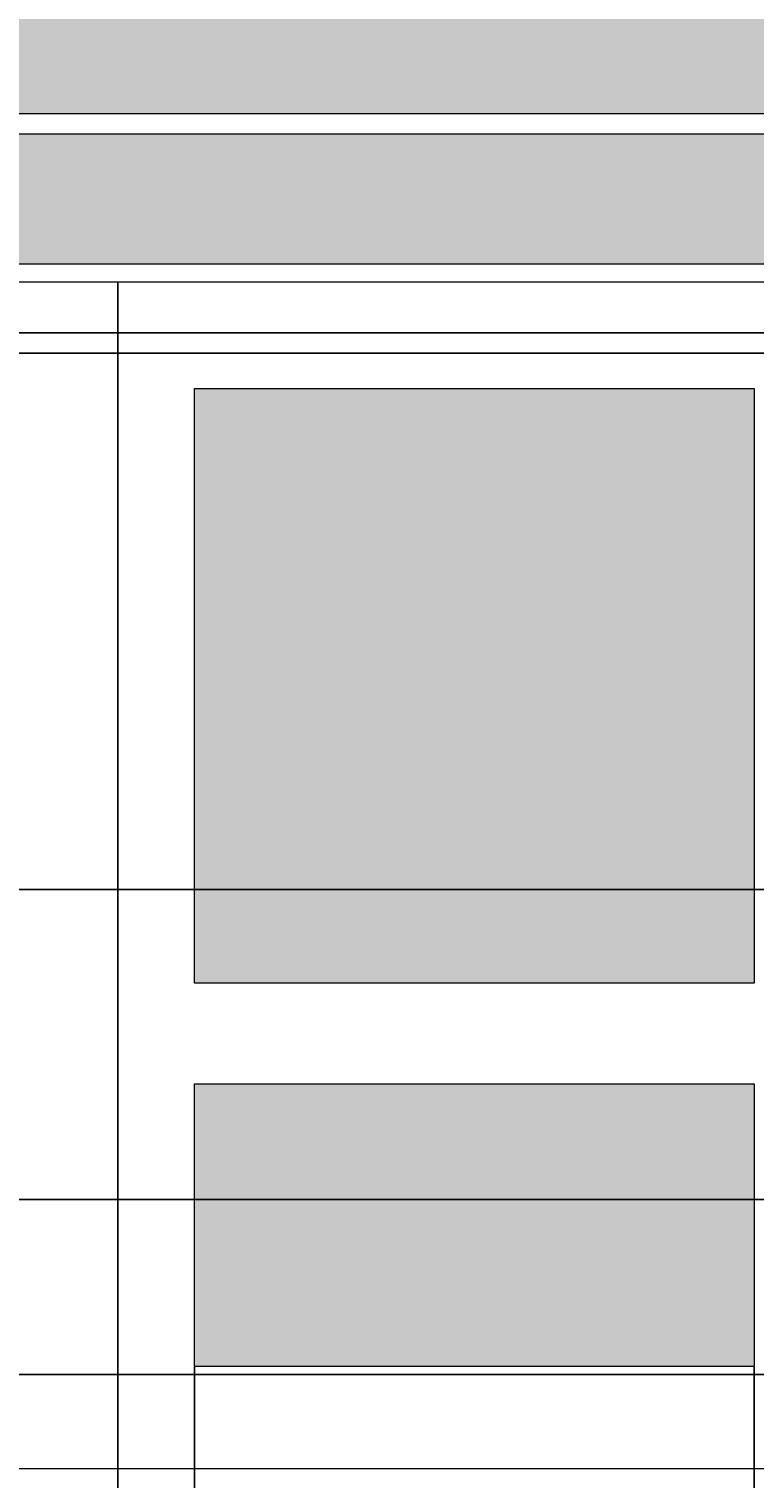
# Model space of a CAD drawing. Units: inches. Extents: x 36 to 594, y 79 to 831.
# Tile 6 of 30: x 319 to 390, y 152 to 294. Entities that reach past the tile are written whole.
import ezdxf

# ---------------------------------------------------------------- set-up
doc = ezdxf.new("R2010")
doc.units = ezdxf.units.IN
doc.header["$MEASUREMENT"] = 0
for name, color, linetype, lineweight in [('A-ANNO-DIMS', 2, 'Continuous', 18), ('A-DOOR', 3, 'Continuous', 18), ('A-ELEV-PATT', 8, 'Continuous', 13)]:
    doc.layers.add(name, color=color, linetype=linetype, lineweight=lineweight)
doc.styles.get("Standard").update_dxf_attribs({"font": 'arial.ttf'})
doc.dimstyles.get("Standard").update_dxf_attribs({"dimtxt": 0.8125, "dimasz": 0.18, "dimexe": 0.18, "dimexo": 0.0625, "dimgap": 0.09, "dimtad": 0, "dimtih": 1, "dimtoh": 1, "dimdec": 4, "dimzin": 0, "dimdsep": 46, "dimlunit": 4, "dimtxsty": 'Standard', "dimcen": 0.09, "dimadec": 0, "dimazin": 0, "dimtfac": 1, "dimtdec": 4, "dimtofl": 0, "dimtmove": 0, "dimatfit": 3, "dimfxl": 1, "dimtolj": 1, "dimtzin": 0, "dimarcsym": 0})

# ---------------------------------------------------------------- blocks, each defined once
blk = doc.blocks.new('*D74')
at = {"layer": 'A-ANNO-DIMS', "color": 0, "lineweight": -2, "transparency": 16777216}
for p, q in [((217.09, 179.42), (592.85, 179.42)), ((592.67, 179.24), (592.67, 171.32)), ((592.67, 162.39), (592.67, 170.31)), ((217.09, 162.21), (592.85, 162.21))]:
    blk.add_line(p, q, dxfattribs=at)
at = {"layer": 'A-ANNO-DIMS', "color": 0, "transparency": 16777216}
for points in [[(592.64, 179.24), (592.7, 179.24), (592.67, 179.42)], [(592.64, 162.39), (592.7, 162.39), (592.67, 162.21)]]:
    blk.add_solid(points, dxfattribs=at)
at = {"layer": 'Defpoints', "color": 0, "transparency": 16777216}
for p in [(217.03, 179.42), (592.67, 179.42), (217.03, 162.21)]:
    blk.add_point(p, dxfattribs=at)
at = {"layer": 'A-ANNO-DIMS', "color": 0, "transparency": 16777216, "insert": (592.67, 170.82), "char_height": 0.812, "attachment_point": 5}
blk.add_mtext('\\A1;17.207', dxfattribs=at)
blk = doc.blocks.new('*D75')
at = {"layer": 'A-ANNO-DIMS', "color": 0, "lineweight": -2, "transparency": 16777216}
for p, q in [((215.09, 262.62), (592.85, 262.62)), ((592.67, 262.44), (592.67, 221.53)), ((592.67, 179.6), (592.67, 220.52)), ((217.09, 179.42), (592.85, 179.42))]:
    blk.add_line(p, q, dxfattribs=at)
at = {"layer": 'A-ANNO-DIMS', "color": 0, "transparency": 16777216}
for points in [[(592.64, 262.44), (592.7, 262.44), (592.67, 262.62)], [(592.64, 179.6), (592.7, 179.6), (592.67, 179.42)]]:
    blk.add_solid(points, dxfattribs=at)
at = {"layer": 'Defpoints', "color": 0, "transparency": 16777216}
for p in [(215.03, 262.62), (592.67, 262.62), (217.03, 179.42)]:
    blk.add_point(p, dxfattribs=at)
at = {"layer": 'A-ANNO-DIMS', "color": 0, "transparency": 16777216, "insert": (592.67, 221.02), "char_height": 0.812, "attachment_point": 5}
blk.add_mtext('\\A1;83.2', dxfattribs=at)
blk = doc.blocks.new('*D76')
at = {"layer": 'A-ANNO-DIMS', "color": 0, "lineweight": -2, "transparency": 16777216}
for p, q in [((217.09, 264.62), (592.85, 264.62)), ((592.67, 264.44), (592.67, 264.12)), ((215.09, 262.62), (592.85, 262.62)), ((592.67, 262.8), (592.67, 263.12))]:
    blk.add_line(p, q, dxfattribs=at)
at = {"layer": 'A-ANNO-DIMS', "color": 0, "transparency": 16777216}
for points in [[(592.64, 264.44), (592.7, 264.44), (592.67, 264.62)], [(592.64, 262.8), (592.7, 262.8), (592.67, 262.62)]]:
    blk.add_solid(points, dxfattribs=at)
at = {"layer": 'Defpoints', "color": 0, "transparency": 16777216}
for p in [(217.03, 264.62), (592.67, 264.62), (215.03, 262.62)]:
    blk.add_point(p, dxfattribs=at)
at = {"layer": 'A-ANNO-DIMS', "color": 0, "transparency": 16777216, "insert": (592.67, 263.62), "char_height": 0.812, "attachment_point": 5}
blk.add_mtext('\\A1;2', dxfattribs=at)
blk = doc.blocks.new('*D77')
at = {"layer": 'A-ANNO-DIMS', "color": 0, "lineweight": -2, "transparency": 16777216}
for p, q in [((151.64, 209.88), (592.85, 209.88)), ((592.67, 209.7), (592.67, 186.55)), ((592.67, 162.39), (592.67, 185.54)), ((156.47, 162.21), (592.85, 162.21))]:
    blk.add_line(p, q, dxfattribs=at)
at = {"layer": 'A-ANNO-DIMS', "color": 0, "transparency": 16777216}
for points in [[(592.64, 209.7), (592.7, 209.7), (592.67, 209.88)], [(592.64, 162.39), (592.7, 162.39), (592.67, 162.21)]]:
    blk.add_solid(points, dxfattribs=at)
at = {"layer": 'Defpoints', "color": 0, "transparency": 16777216}
for p in [(151.58, 209.88), (156.41, 162.21), (592.67, 162.21)]:
    blk.add_point(p, dxfattribs=at)
at = {"layer": 'A-ANNO-DIMS', "color": 0, "transparency": 16777216, "insert": (592.67, 186.05), "char_height": 0.812, "attachment_point": 5}
blk.add_mtext('\\A1;47.67', dxfattribs=at)
blk = doc.blocks.new('*D80')
at = {"layer": 'A-ANNO-DIMS', "color": 0, "lineweight": -2, "transparency": 16777216}
for p, q in [((317.35, 162.93), (317.35, 79.53)), ((327.79, 152.87), (327.79, 79.53)), ((317.53, 79.71), (320.83, 79.71)), ((327.61, 79.71), (324.31, 79.71))]:
    blk.add_line(p, q, dxfattribs=at)
at = {"layer": 'A-ANNO-DIMS', "color": 0, "transparency": 16777216}
for points in [[(317.53, 79.74), (317.53, 79.68), (317.35, 79.71)], [(327.61, 79.74), (327.61, 79.68), (327.79, 79.71)]]:
    blk.add_solid(points, dxfattribs=at)
at = {"layer": 'Defpoints', "color": 0, "transparency": 16777216}
for p in [(317.35, 162.99), (327.79, 152.93), (327.79, 79.71)]:
    blk.add_point(p, dxfattribs=at)
at = {"layer": 'A-ANNO-DIMS', "color": 0, "transparency": 16777216, "insert": (322.57, 79.71), "char_height": 0.812, "attachment_point": 5}
blk.add_mtext('\\A1;10.436', dxfattribs=at)
blk = doc.blocks.new('*D81')
at = {"layer": 'A-ANNO-DIMS', "color": 0, "lineweight": -2, "transparency": 16777216}
for p, q in [((335.35, 162.93), (335.35, 79.53)), ((327.79, 152.87), (327.79, 79.53)), ((327.97, 79.71), (330.43, 79.71)), ((335.17, 79.71), (332.71, 79.71))]:
    blk.add_line(p, q, dxfattribs=at)
at = {"layer": 'A-ANNO-DIMS', "color": 0, "transparency": 16777216}
for points in [[(327.97, 79.74), (327.97, 79.68), (327.79, 79.71)], [(335.17, 79.74), (335.17, 79.68), (335.35, 79.71)]]:
    blk.add_solid(points, dxfattribs=at)
at = {"layer": 'Defpoints', "color": 0, "transparency": 16777216}
for p in [(335.35, 162.99), (327.79, 152.93), (335.35, 79.71)]:
    blk.add_point(p, dxfattribs=at)
at = {"layer": 'A-ANNO-DIMS', "color": 0, "transparency": 16777216, "insert": (331.57, 79.71), "char_height": 0.812, "attachment_point": 5}
blk.add_mtext('\\A1;7.56', dxfattribs=at)
blk = doc.blocks.new('*D82')
at = {"layer": 'A-ANNO-DIMS', "color": 0, "lineweight": -2, "transparency": 16777216}
for p, q in [((335.35, 162.93), (335.35, 79.53)), ((390.39, 162.93), (390.39, 79.53)), ((335.53, 79.71), (361.41, 79.71)), ((390.21, 79.71), (364.33, 79.71))]:
    blk.add_line(p, q, dxfattribs=at)
at = {"layer": 'A-ANNO-DIMS', "color": 0, "transparency": 16777216}
for points in [[(335.53, 79.74), (335.53, 79.68), (335.35, 79.71)], [(390.21, 79.74), (390.21, 79.68), (390.39, 79.71)]]:
    blk.add_solid(points, dxfattribs=at)
at = {"layer": 'Defpoints', "color": 0, "transparency": 16777216}
for p in [(335.35, 162.99), (390.39, 162.99), (390.39, 79.71)]:
    blk.add_point(p, dxfattribs=at)
at = {"layer": 'A-ANNO-DIMS', "color": 0, "transparency": 16777216, "insert": (362.87, 79.71), "char_height": 0.812, "attachment_point": 5}
blk.add_mtext('\\A1;55.04', dxfattribs=at)

msp = doc.modelspace()

# ---------------------------------------------------------------- hatches: boundary and pattern name
at = {"layer": 'A-ELEV-PATT'}
h = msp.add_hatch(color=256, dxfattribs=at)
h.dxf.hatch_style = 1
h.paths.add_polyline_path([(398.0873, 796.0465), (269.3592, 796.0465), (269.3592, 770.1455), (397.8159, 770.1455)])
h.paths.add_polyline_path([(397.7518, 764.0341), (269.3592, 764.0341), (269.3592, 630.0394), (341.8367, 630.0394), (341.8367, 720.595), (335.0881, 728.3699), (329.982, 735.3373), (345.3661, 727.7743), (397.1052, 702.3389)])
h.paths.add_polyline_path([(341.8367, 594.2124), (201.4189, 594.2124), (201.4189, 475.4136), (232.8216, 475.4136), (232.8216, 524.6037), (341.8367, 524.6037)])
h.paths.add_polyline_path([(177.525, 594.2124), (118.7598, 594.2124), (118.7598, 450.2124), (177.525, 450.2124)])
h.paths.add_polyline_path([(424.4958, 594.2124), (365.7306, 594.2124), (365.7306, 450.2124), (424.4958, 450.2124)])
h.paths.add_polyline_path([(241.3553, 404.2737), (355.8569, 404.2737), (355.8569, 355.0836), (424.5492, 355.0836), (424.5492, 425.7333), (118.7598, 426.2844), (118.7598, 355.0836), (241.3553, 355.0836)])
h.paths.add_polyline_path([(448.3898, 306.2124), (217.0273, 306.2124), (217.0273, 142.2124), (254.0293, 142.2124), (254.0293, 150.9347), (254.0293, 286.1802), (401.5491, 286.1802), (401.5491, 150.9347), (401.5491, 142.2124), (448.3898, 142.2124)])
h.paths.add_polyline_path([(448.3898, 142.2124), (401.5491, 142.2124), (217.0273, 142.2124), (217.0273, 114.2124), (448.3898, 114.2124)])
h.paths.add_polyline_path([(217.0273, 306.2124), (174.7353, 306.2124), (94.8658, 306.2124), (94.8658, 162.2124), (103.3368, 162.2124), (103.3368, 264.6224), (103.3368, 286.1802), (217.0273, 286.1802)])
h = msp.add_hatch(color=256, dxfattribs=at)
h.dxf.hatch_style = 1
h.set_gradient(color1=(0, 255, 255), color2=(16, 86, 137))
h.paths.add_polyline_path([(341.8367, 524.6037), (260.5056, 524.6037), (260.5056, 513.1224), (341.8367, 513.1224)])
h.paths.add_polyline_path([(341.8367, 511.1224), (260.5056, 511.1224), (260.5056, 475.4136), (341.8367, 475.4136)])
h.paths.add_polyline_path([(258.5056, 524.6037), (232.8216, 524.6037), (232.8216, 513.1224), (258.5056, 513.1224)])
h.paths.add_polyline_path([(355.8569, 404.2737), (269.0393, 404.2737), (269.0393, 392.7924), (355.8569, 392.7924)])
h.paths.add_polyline_path([(267.0393, 404.2737), (241.3553, 404.2737), (241.3553, 392.7924), (267.0393, 392.7924)])
h.paths.add_polyline_path([(355.8569, 390.7924), (269.0393, 390.7924), (269.0393, 355.0836), (355.8569, 355.0836)])
h.paths.add_polyline_path([(399.5491, 284.1802), (256.0293, 284.1802), (256.0293, 271.378), (399.5491, 271.378)])
h.paths.add_polyline_path([(317.3533, 259.1243), (262.3169, 259.1243), (262.3169, 200.6645), (317.3533, 200.6645)])
h.paths.add_polyline_path([(390.386, 259.1243), (335.3496, 259.1243), (335.3496, 200.6645), (390.386, 200.6645)])
h.paths.add_polyline_path([(390.386, 190.7697), (335.3496, 190.7697), (335.3496, 162.9881), (390.386, 162.9881)])
h.paths.add_polyline_path([(317.3533, 190.7697), (262.3169, 190.7697), (262.3169, 162.9881), (317.3533, 162.9881)])
h.paths.add_polyline_path([(215.0273, 262.6224), (158.4069, 262.6224), (158.4069, 181.4195), (215.0273, 181.4195)])
h.paths.add_polyline_path([(215.0273, 284.1802), (105.3368, 284.1802), (105.3368, 266.6224), (215.0273, 266.6224)])

# ---------------------------------------------------------------- linework, layer by layer
at = {"layer": 'A-DOOR'}
msp.add_line((256.0293, 271.378), (399.5491, 271.378), dxfattribs=at)
for points in [[(254.0293, 286.1802), (401.5491, 286.1802), (401.5491, 150.9347), (254.0293, 150.9347)], [(256.0293, 284.1802), (399.5491, 284.1802), (399.5491, 152.9347), (256.0293, 152.9347)], [(256.0293, 269.6084), (327.7892, 269.6084), (327.7892, 152.9347), (256.0293, 152.9347)], [(327.7892, 269.6084), (399.5491, 269.6084), (399.5491, 152.9347), (327.7892, 152.9347)], [(335.3496, 259.1243), (390.386, 259.1243), (390.386, 200.6645), (335.3496, 200.6645)], [(335.3496, 190.7697), (390.386, 190.7697), (390.386, 162.9881), (335.3496, 162.9881)]]:
    msp.add_lwpolyline(points, close=True, dxfattribs=at)

# ---------------------------------------------------------------- dimensions: what is measured, and where the dimension line sits
at = {"layer": 'A-ANNO-DIMS'}
for base, p1, p2, override, picture, middle in [((592.6689, 264.6224), (215.0273, 262.6224), (217.0273, 264.6224), {"dimdec": 0, "dimlfac": 1, "dimrnd": 0, "dimzin": 0, "dimdsep": 46, "dimlunit": 2}, '*D76', (592.6689, 263.6224)), ((592.6689, 262.6224), (217.0273, 179.4195), (215.0273, 262.6224), {"dimdec": 1, "dimlfac": 1, "dimrnd": 0, "dimzin": 0, "dimdsep": 46, "dimlunit": 2}, '*D75', (592.6689, 221.021)), ((592.6689, 162.2124), (151.5799, 209.8823), (156.4069, 162.2124), {"dimdec": 2, "dimlfac": 1, "dimrnd": 0, "dimzin": 0, "dimdsep": 46, "dimlunit": 2}, '*D77', (592.6689, 186.0473)), ((592.6689, 179.4195), (217.0273, 162.2124), (217.0273, 179.4195), {"dimdec": 3, "dimlfac": 1, "dimrnd": 0, "dimzin": 0, "dimdsep": 46, "dimlunit": 2}, '*D74', (592.6689, 170.8159))]:
    dim = msp.add_linear_dim(base=base, p1=p1, p2=p2, angle=90, dimstyle='Standard', override=override, dxfattribs=at)
    dim.commit()
    dim.dimension.update_dxf_attribs({"geometry": picture, "text_midpoint": middle})
for base, p1, p2, override, picture, middle in [((327.7892, 79.7124), (317.3533, 162.9881), (327.7892, 152.9347), {"dimdec": 3, "dimlfac": 1, "dimrnd": 0, "dimzin": 0, "dimdsep": 46, "dimlunit": 2}, '*D80', (322.5712, 79.7124)), ((335.3496, 79.7124), (327.7892, 152.9347), (335.3496, 162.9881), {"dimdec": 2, "dimlfac": 1, "dimrnd": 0, "dimzin": 0, "dimdsep": 46, "dimlunit": 2}, '*D81', (331.5694, 79.7124)), ((390.386, 79.7124), (335.3496, 162.9881), (390.386, 162.9881), {"dimdec": 2, "dimlfac": 1, "dimrnd": 0, "dimzin": 0, "dimdsep": 46, "dimlunit": 2}, '*D82', (362.8678, 79.7124))]:
    dim = msp.add_linear_dim(base=base, p1=p1, p2=p2, dimstyle='Standard', override=override, dxfattribs=at)
    dim.commit()
    dim.dimension.update_dxf_attribs({"geometry": picture, "text_midpoint": middle})

doc.saveas('drawing.dxf')
